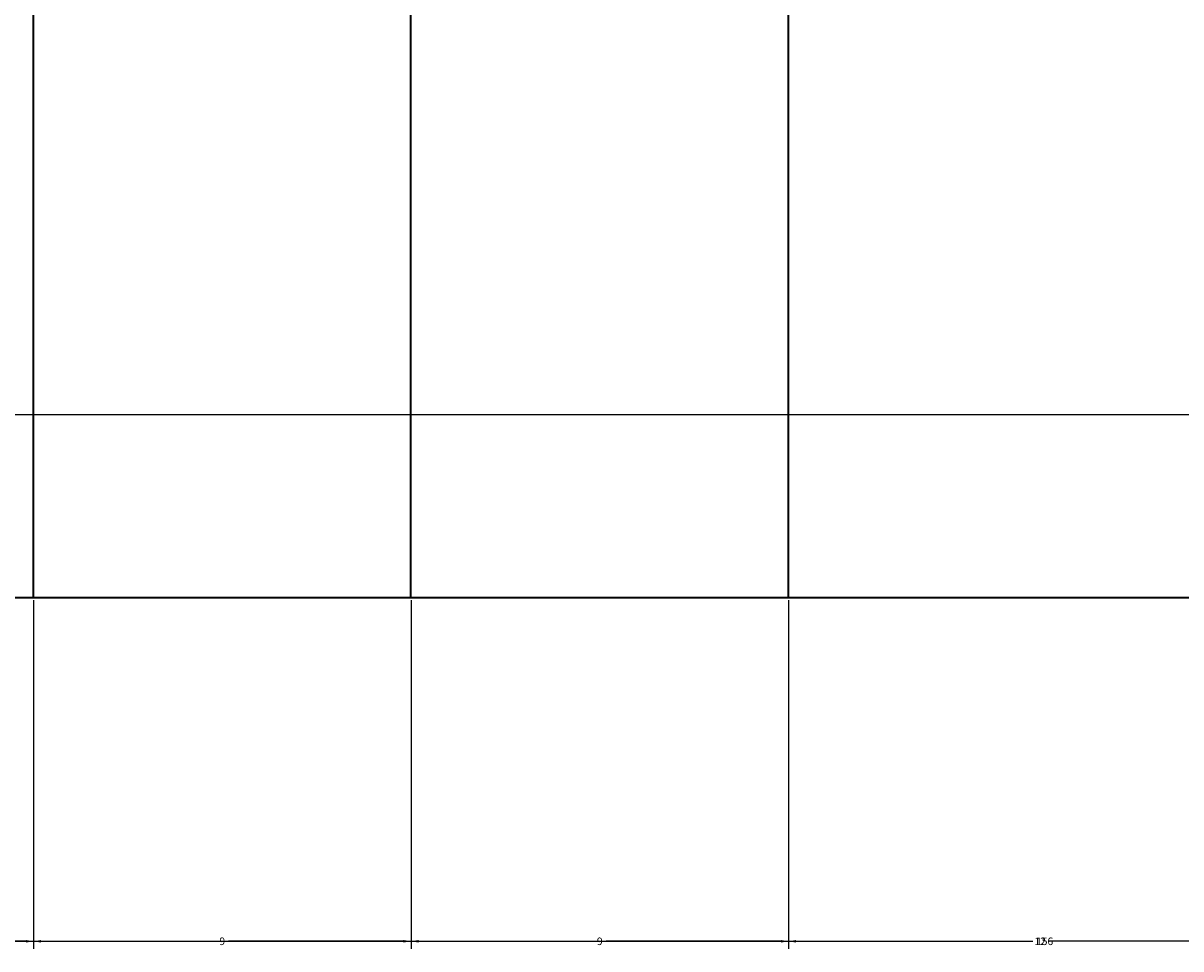
# Model space of a CAD drawing. Units: inches. Extents: x 27 to 200, y -50 to 102.
# Tile 8 of 26: x 89 to 117, y -25 to -3. Entities that reach past the tile are written whole.
import ezdxf

# ---------------------------------------------------------------- set-up
doc = ezdxf.new("R2010")
doc.units = ezdxf.units.IN
doc.header["$MEASUREMENT"] = 0
doc.layers.add('A-ANNO-DIMS', color=2, linetype='Continuous', lineweight=18)
doc.layers.add('A-ELEV', color=7, linetype='Continuous', lineweight=35)
doc.styles.get("Standard").update_dxf_attribs({"font": 'arial.ttf'})
doc.dimstyles.get("Standard").update_dxf_attribs({"dimtxt": 0.18, "dimasz": 0.18, "dimexe": 0.18, "dimexo": 0.0625, "dimgap": 0.09, "dimtad": 0, "dimtih": 1, "dimtoh": 1, "dimdec": 4, "dimzin": 0, "dimdsep": 46, "dimtxsty": 'Standard', "dimcen": 0.09, "dimadec": 0, "dimazin": 0, "dimtfac": 1, "dimtdec": 4, "dimtofl": 0, "dimtmove": 0, "dimatfit": 3, "dimfxl": 1, "dimtolj": 1, "dimtzin": 0, "dimarcsym": 0})

# ---------------------------------------------------------------- blocks, each defined once
blk = doc.blocks.new('*D23')
at = {"layer": 'A-ANNO-DIMS', "color": 0, "lineweight": -2, "transparency": 16777216}
for p, q in [((35.417, -16.832), (35.417, -25.149)), ((191.417, -16.832), (191.417, -25.149)), ((35.597, -24.969), (113.137, -24.969)), ((191.237, -24.969), (113.697, -24.969))]:
    blk.add_line(p, q, dxfattribs=at)
at = {"layer": 'A-ANNO-DIMS', "color": 0, "transparency": 16777216}
for points in [[(35.597, -24.939), (35.597, -24.999), (35.417, -24.969)], [(191.237, -24.939), (191.237, -24.999), (191.417, -24.969)]]:
    blk.add_solid(points, dxfattribs=at)
at = {"layer": 'Defpoints', "color": 0, "transparency": 16777216}
for p in [(35.417, -16.769), (191.417, -16.769), (191.417, -24.969)]:
    blk.add_point(p, dxfattribs=at)
at = {"layer": 'A-ANNO-DIMS', "color": 0, "transparency": 16777216, "insert": (113.417, -24.969), "char_height": 0.18, "attachment_point": 5}
blk.add_mtext('\\A1;156', dxfattribs=at)
blk = doc.blocks.new('*D33')
at = {"layer": 'A-ANNO-DIMS', "color": 0, "lineweight": -2, "transparency": 16777216}
for p, q in [((84.417, -16.832), (84.417, -25.149)), ((89.312, -16.832), (89.312, -25.149)), ((84.597, -24.969), (86.466, -24.969)), ((89.132, -24.969), (87.262, -24.969))]:
    blk.add_line(p, q, dxfattribs=at)
at = {"layer": 'A-ANNO-DIMS', "color": 0, "transparency": 16777216}
for points in [[(84.597, -24.939), (84.597, -24.999), (84.417, -24.969)], [(89.132, -24.939), (89.132, -24.999), (89.312, -24.969)]]:
    blk.add_solid(points, dxfattribs=at)
at = {"layer": 'Defpoints', "color": 0, "transparency": 16777216}
for p in [(84.417, -16.769), (89.312, -16.769), (89.312, -24.969)]:
    blk.add_point(p, dxfattribs=at)
at = {"layer": 'A-ANNO-DIMS', "color": 0, "transparency": 16777216, "insert": (86.864, -24.969), "char_height": 0.18, "attachment_point": 5}
blk.add_mtext('\\A1;4.895', dxfattribs=at)
blk = doc.blocks.new('*D34')
at = {"layer": 'A-ANNO-DIMS', "color": 0, "lineweight": -2, "transparency": 16777216}
for p, q in [((89.312, -16.832), (89.312, -25.149)), ((98.312, -16.832), (98.312, -25.149)), ((89.492, -24.969), (93.663, -24.969)), ((98.132, -24.969), (93.961, -24.969))]:
    blk.add_line(p, q, dxfattribs=at)
at = {"layer": 'A-ANNO-DIMS', "color": 0, "transparency": 16777216}
for points in [[(89.492, -24.939), (89.492, -24.999), (89.312, -24.969)], [(98.132, -24.939), (98.132, -24.999), (98.312, -24.969)]]:
    blk.add_solid(points, dxfattribs=at)
at = {"layer": 'Defpoints', "color": 0, "transparency": 16777216}
for p in [(89.312, -16.769), (98.312, -16.769), (98.312, -24.969)]:
    blk.add_point(p, dxfattribs=at)
at = {"layer": 'A-ANNO-DIMS', "color": 0, "transparency": 16777216, "insert": (93.812, -24.969), "char_height": 0.18, "attachment_point": 5}
blk.add_mtext('\\A1;9', dxfattribs=at)
blk = doc.blocks.new('*D35')
at = {"layer": 'A-ANNO-DIMS', "color": 0, "lineweight": -2, "transparency": 16777216}
for p, q in [((98.312, -16.832), (98.312, -25.149)), ((107.312, -16.832), (107.312, -25.149)), ((98.492, -24.969), (102.663, -24.969)), ((107.132, -24.969), (102.961, -24.969))]:
    blk.add_line(p, q, dxfattribs=at)
at = {"layer": 'A-ANNO-DIMS', "color": 0, "transparency": 16777216}
for points in [[(98.492, -24.939), (98.492, -24.999), (98.312, -24.969)], [(107.132, -24.939), (107.132, -24.999), (107.312, -24.969)]]:
    blk.add_solid(points, dxfattribs=at)
at = {"layer": 'Defpoints', "color": 0, "transparency": 16777216}
for p in [(98.312, -16.769), (107.312, -16.769), (107.312, -24.969)]:
    blk.add_point(p, dxfattribs=at)
at = {"layer": 'A-ANNO-DIMS', "color": 0, "transparency": 16777216, "insert": (102.812, -24.969), "char_height": 0.18, "attachment_point": 5}
blk.add_mtext('\\A1;9', dxfattribs=at)
blk = doc.blocks.new('*D36')
at = {"layer": 'A-ANNO-DIMS', "color": 0, "lineweight": -2, "transparency": 16777216}
for p, q in [((107.312, -16.832), (107.312, -25.149)), ((119.312, -16.832), (119.312, -25.149)), ((107.492, -24.969), (113.102, -24.969)), ((119.132, -24.969), (113.521, -24.969))]:
    blk.add_line(p, q, dxfattribs=at)
at = {"layer": 'A-ANNO-DIMS', "color": 0, "transparency": 16777216}
for points in [[(107.492, -24.939), (107.492, -24.999), (107.312, -24.969)], [(119.132, -24.939), (119.132, -24.999), (119.312, -24.969)]]:
    blk.add_solid(points, dxfattribs=at)
at = {"layer": 'Defpoints', "color": 0, "transparency": 16777216}
for p in [(107.312, -16.769), (119.312, -16.769), (119.312, -24.969)]:
    blk.add_point(p, dxfattribs=at)
at = {"layer": 'A-ANNO-DIMS', "color": 0, "transparency": 16777216, "insert": (113.312, -24.969), "char_height": 0.18, "attachment_point": 5}
blk.add_mtext('\\A1;12', dxfattribs=at)
blk = doc.blocks.new('*D48')
at = {"layer": 'A-ANNO-DIMS', "color": 0, "lineweight": -2, "transparency": 16777216}
for p, q in [((84.479, 44.926), (199.797, 44.926)), ((199.617, 44.746), (199.617, 14.26)), ((199.617, -16.589), (199.617, 13.897)), ((84.479, -16.769), (199.797, -16.769))]:
    blk.add_line(p, q, dxfattribs=at)
at = {"layer": 'A-ANNO-DIMS', "color": 0, "transparency": 16777216}
for points in [[(199.587, 44.746), (199.647, 44.746), (199.617, 44.926)], [(199.587, -16.589), (199.647, -16.589), (199.617, -16.769)]]:
    blk.add_solid(points, dxfattribs=at)
at = {"layer": 'Defpoints', "color": 0, "transparency": 16777216}
for p in [(84.417, 44.926), (199.617, 44.926), (84.417, -16.769)]:
    blk.add_point(p, dxfattribs=at)
at = {"layer": 'A-ANNO-DIMS', "color": 0, "transparency": 16777216, "insert": (199.617, 14.079), "char_height": 0.18, "attachment_point": 5}
blk.add_mtext('\\A1;61.7', dxfattribs=at)
blk = doc.blocks.new('*D56')
at = {"layer": 'A-ANNO-DIMS', "color": 0, "lineweight": -2, "transparency": 16777216}
for p, q in [((121.225, 5.878), (27.037, 5.878)), ((27.217, 5.698), (27.217, -3.085)), ((27.217, -12.231), (27.217, -3.448)), ((121.225, -12.411), (27.037, -12.411))]:
    blk.add_line(p, q, dxfattribs=at)
at = {"layer": 'A-ANNO-DIMS', "color": 0, "transparency": 16777216}
for points in [[(27.187, 5.698), (27.247, 5.698), (27.217, 5.878)], [(27.187, -12.231), (27.247, -12.231), (27.217, -12.411)]]:
    blk.add_solid(points, dxfattribs=at)
at = {"layer": 'Defpoints', "color": 0, "transparency": 16777216}
for p in [(27.217, 5.878), (121.288, 5.878), (121.288, -12.411)]:
    blk.add_point(p, dxfattribs=at)
at = {"layer": 'A-ANNO-DIMS', "color": 0, "transparency": 16777216, "insert": (27.217, -3.267), "char_height": 0.18, "attachment_point": 5}
blk.add_mtext('\\A1;18.29', dxfattribs=at)
blk = doc.blocks.new('*D69')
at = {"layer": 'A-ANNO-DIMS', "color": 0, "lineweight": -2, "transparency": 16777216}
for p, q in [((121.225, -12.411), (27.037, -12.411)), ((27.217, -12.591), (27.217, -14.408)), ((27.217, -16.589), (27.217, -14.772)), ((119.249, -16.769), (27.037, -16.769))]:
    blk.add_line(p, q, dxfattribs=at)
at = {"layer": 'A-ANNO-DIMS', "color": 0, "transparency": 16777216}
for points in [[(27.187, -12.591), (27.247, -12.591), (27.217, -12.411)], [(27.187, -16.589), (27.247, -16.589), (27.217, -16.769)]]:
    blk.add_solid(points, dxfattribs=at)
at = {"layer": 'Defpoints', "color": 0, "transparency": 16777216}
for p in [(27.217, -12.411), (121.288, -12.411), (119.312, -16.769)]:
    blk.add_point(p, dxfattribs=at)
at = {"layer": 'A-ANNO-DIMS', "color": 0, "transparency": 16777216, "insert": (27.217, -14.59), "char_height": 0.18, "attachment_point": 5}
blk.add_mtext('\\A1;4.358', dxfattribs=at)

msp = doc.modelspace()

# ---------------------------------------------------------------- linework, layer by layer
at = {"layer": 'A-ELEV'}
for p, q in [((89.3118, -16.7693), (89.3118, 19.2307)), ((98.3118, -16.7693), (98.3118, 16.2105)), ((107.3118, -16.7693), (107.3118, 16.1904)), ((35.4169, -16.7693), (191.4169, -16.7693))]:
    msp.add_line(p, q, dxfattribs=at)

# ---------------------------------------------------------------- dimensions: what is measured, and where the dimension line sits
at = {"layer": 'A-ANNO-DIMS'}
for base, p1, p2, override, picture, middle in [((199.6169, 44.9264), (84.4169, -16.7693), (84.4169, 44.9264), {"dimdec": 1, "dimlfac": 1, "dimrnd": 0, "dimzin": 0, "dimdsep": 46, "dimlunit": 2}, '*D48', (199.6169, 14.0786)), ((27.2169, 5.8779), (121.2876, -12.411), (121.2876, 5.8779), {"dimdec": 2, "dimlfac": 1, "dimrnd": 0, "dimzin": 0, "dimdsep": 46, "dimlunit": 2}, '*D56', (27.2169, -3.2665)), ((27.2169, -12.411), (119.3118, -16.7693), (121.2876, -12.411), {"dimdec": 3, "dimlfac": 1, "dimrnd": 0, "dimzin": 0, "dimdsep": 46, "dimlunit": 2}, '*D69', (27.2169, -14.5901))]:
    dim = msp.add_linear_dim(base=base, p1=p1, p2=p2, angle=90, dimstyle='Standard', override=override, dxfattribs=at)
    dim.commit()
    dim.dimension.update_dxf_attribs({"geometry": picture, "text_midpoint": middle})
for base, p1, p2, override, picture, middle in [((191.4169, -24.9693), (35.4169, -16.7693), (191.4169, -16.7693), {"dimdec": 0, "dimlfac": 1, "dimrnd": 0, "dimzin": 0, "dimdsep": 46, "dimlunit": 2}, '*D23', (113.4169, -24.9693)), ((89.3118, -24.9693), (84.4169, -16.7693), (89.3118, -16.7693), {"dimdec": 3, "dimlfac": 1, "dimrnd": 0, "dimzin": 0, "dimdsep": 46, "dimlunit": 2}, '*D33', (86.8644, -24.9693)), ((98.3118, -24.9693), (89.3118, -16.7693), (98.3118, -16.7693), {"dimdec": 0, "dimlfac": 1, "dimrnd": 0, "dimzin": 0, "dimdsep": 46, "dimlunit": 2}, '*D34', (93.8118, -24.9693)), ((107.3118, -24.9693), (98.3118, -16.7693), (107.3118, -16.7693), {"dimdec": 0, "dimlfac": 1, "dimrnd": 0, "dimzin": 0, "dimdsep": 46, "dimlunit": 2}, '*D35', (102.8118, -24.9693)), ((119.3118, -24.9693), (107.3118, -16.7693), (119.3118, -16.7693), {"dimdec": 0, "dimlfac": 1, "dimrnd": 0, "dimzin": 0, "dimdsep": 46, "dimlunit": 2}, '*D36', (113.3118, -24.9693))]:
    dim = msp.add_linear_dim(base=base, p1=p1, p2=p2, dimstyle='Standard', override=override, dxfattribs=at)
    dim.commit()
    dim.dimension.update_dxf_attribs({"geometry": picture, "text_midpoint": middle})

doc.saveas('drawing.dxf')
